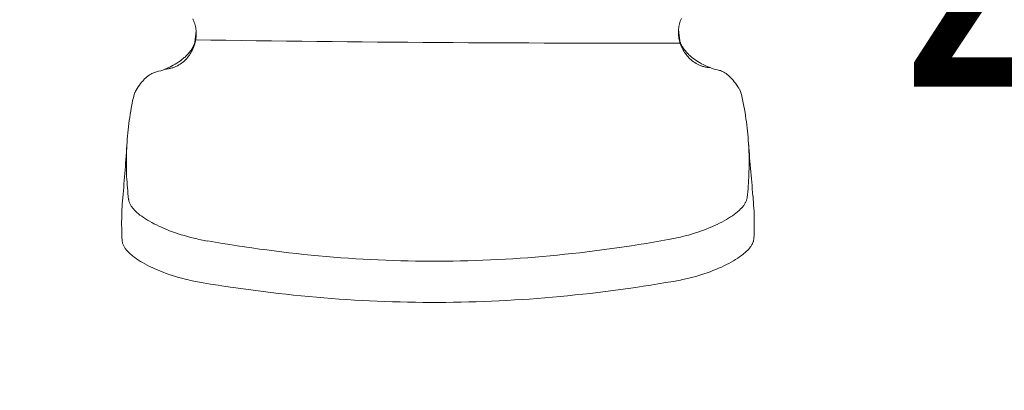
# Model space of a CAD drawing. Units: inches. Extents: x -466983 to 1020, y 324 to 318697.
# Tile 35 of 97: x 867.6 to 887.72, y 734.38 to 741.96. Entities that reach past the tile are written whole.
import ezdxf

# ---------------------------------------------------------------- set-up
doc = ezdxf.new("R2010")
doc.units = ezdxf.units.IN
doc.header["$MEASUREMENT"] = 0
for name, color, linetype, lineweight in [('A-ANNO-DIMS', 2, 'Continuous', 18), ('A-FLOR-PATT', 252, 'Continuous', 13), ('A-FURN', 8, 'Continuous', 18)]:
    doc.layers.add(name, color=color, linetype=linetype, lineweight=lineweight)
doc.styles.get("Standard").update_dxf_attribs({"font": 'arial.ttf'})
doc.dimstyles.get("Standard").update_dxf_attribs({"dimtxt": 6, "dimasz": 4, "dimexe": 3, "dimexo": 3, "dimgap": 0.09, "dimtad": 0, "dimtih": 1, "dimtoh": 1, "dimdec": 1, "dimzin": 0, "dimdsep": 46, "dimlunit": 3, "dimtxsty": 'Standard', "dimcen": 0.09, "dimadec": 0, "dimazin": 0, "dimtfac": 1, "dimtdec": 1, "dimtofl": 0, "dimtmove": 0, "dimatfit": 3, "dimfxl": 1, "dimtolj": 1, "dimtzin": 0, "dimarcsym": 0})

# ---------------------------------------------------------------- blocks, each defined once
blk = doc.blocks.new('Office Chairs')
at = {"ltscale": 60}
for p, q in [((3701, 927.5), (3701.6, 926.1)), ((3701.6, 926.1), (3702.2, 924.7)), ((3702.2, 924.7), (3702.7, 923.3)), ((3702.7, 923.3), (3703.2, 921.9)), ((4219.7, 923.5), (4219.4, 922.1)), ((4220.2, 924.9), (4219.7, 923.5)), ((4220.7, 926.3), (4220.2, 924.9)), ((4221.3, 927.7), (4220.7, 926.3)), ((3703.2, 921.9), (3703.6, 920.5)), ((3703.6, 920.5), (3703.9, 919.1)), ((3703.9, 919.1), (3704.2, 917.7)), ((3704.2, 917.7), (3704.4, 916.2)), ((3704.4, 916.2), (3704.6, 914.8)), ((3704.6, 914.8), (3704.7, 913.4)), ((3704.7, 913.8), (3704.7, 909.7)), ((3704.7, 913.4), (3704.7, 912)), ((4218.3, 914.9), (4218.2, 913.5)), ((4218.2, 913.5), (4218.2, 912.8)), ((4218.2, 912.8), (4218.2, 912.7)), ((4218.4, 916.4), (4218.3, 914.9)), ((4218.3, 915.2), (4218.3, 911.3)), ((4218.5, 917.8), (4218.4, 916.4)), ((4218.8, 919.2), (4218.5, 917.8)), ((4219, 920.7), (4218.8, 919.2)), ((4219.4, 922.1), (4219, 920.7)), ((3703, 901.2), (3703.2, 902.1)), ((3703.2, 902.1), (3703.2, 902.3)), ((3703.2, 902.3), (3703.2, 902.3)), ((3703.3, 900.6), (3703.6, 902.1)), ((3703.6, 902.1), (3704, 903.5)), ((3704, 903.5), (3704.2, 904.9)), ((3704.2, 904.9), (3704.4, 906.4)), ((3704.4, 906.4), (3704.6, 907.9)), ((3704.6, 907.9), (3704.7, 908.6)), ((3704.7, 912), (3704.8, 911.2)), ((3704.7, 909.7), (3704.7, 908.6)), ((4218.3, 911.3), (4218.3, 910.2)), ((4218.4, 909.4), (4218.3, 910.2)), ((4218.6, 908), (4218.4, 909.4)), ((4218.8, 906.5), (4218.6, 908)), ((4219.1, 905.1), (4218.8, 906.5)), ((4219.4, 903.6), (4219.1, 905.1)), ((4219.8, 902.2), (4219.4, 903.6)), ((4219.8, 903.7), (4219.8, 904)), ((4219.8, 904), (4219.8, 904)), ((4220, 902.8), (4219.8, 903.7)), ((4220.2, 900.8), (4219.8, 902.2)), ((4220.3, 901.9), (4220, 902.8)), ((4220.5, 901.4), (4220.3, 901.9)), ((3697.4, 891.4), (3696.7, 890.6)), ((3698.1, 892.3), (3697.4, 891.4)), ((3698.8, 893.2), (3698.1, 892.3)), ((3698.4, 890), (3699.2, 891.2)), ((3699.4, 894), (3698.8, 893.2)), ((3699.2, 891.2), (3699.9, 892.5)), ((3700, 895), (3699.4, 894)), ((3699.9, 892.5), (3700.6, 893.8)), ((3700.6, 895.9), (3700, 895)), ((3701.1, 896.8), (3700.6, 895.9)), ((3700.6, 893.8), (3701.2, 895.1)), ((3701.6, 897.8), (3701.1, 896.8)), ((3701.2, 895.1), (3701.8, 896.5)), ((3702.1, 898.8), (3701.6, 897.8)), ((3701.8, 896.5), (3702.3, 897.9)), ((3702.6, 899.8), (3702.1, 898.8)), ((3702.3, 897.9), (3702.8, 899.2)), ((3702.6, 899.8), (3702.7, 900.3)), ((3702.7, 900.3), (3703, 901.2)), ((3702.8, 899.2), (3703.3, 900.6)), ((4220.7, 899.4), (4220.2, 900.8)), ((4220.5, 901.4), (4220.9, 900.4)), ((4221.3, 898.1), (4220.7, 899.4)), ((4220.9, 900.4), (4221.4, 899.4)), ((4221.9, 896.7), (4221.3, 898.1)), ((4221.4, 899.4), (4221.9, 898.4)), ((4221.9, 898.4), (4222.5, 897.5)), ((4222.5, 895.4), (4221.9, 896.7)), ((4222.5, 897.5), (4223.1, 896.6)), ((4223.2, 894.1), (4222.5, 895.4)), ((4223.1, 896.6), (4223.7, 895.7)), ((4223.9, 892.8), (4223.2, 894.1)), ((4223.7, 895.7), (4224.3, 894.8)), ((4224.7, 891.6), (4223.9, 892.8)), ((4224.3, 894.8), (4225, 893.9)), ((4225.6, 890.4), (4224.7, 891.6)), ((4225, 893.9), (4225.7, 893.1)), ((4225.7, 893.1), (4226.4, 892.2)), ((4226.4, 892.2), (4227.1, 891.4)), ((4227.1, 891.4), (4227.9, 890.6)), ((3686.1, 881.4), (3684.2, 880.2)), ((3687.9, 882.6), (3686.1, 881.4)), ((3689.6, 883.9), (3687.9, 882.6)), ((3689, 880), (3690.3, 881)), ((3691.3, 885.3), (3689.6, 883.9)), ((3690.3, 881), (3691.5, 882)), ((3692.1, 886), (3691.3, 885.3)), ((3691.5, 882), (3692.6, 883)), ((3692.9, 886.7), (3692.1, 886)), ((3692.6, 883), (3693.7, 884.1)), ((3693.7, 887.5), (3692.9, 886.7)), ((3694.5, 888.2), (3693.7, 887.5)), ((3693.7, 884.1), (3694.8, 885.2)), ((3695.3, 889), (3694.5, 888.2)), ((3694.8, 885.2), (3695.8, 886.4)), ((3696, 889.8), (3695.3, 889)), ((3695.8, 886.4), (3696.7, 887.6)), ((3696.7, 890.6), (3696, 889.8)), ((3696.7, 887.6), (3697.6, 888.8)), ((3697.6, 888.8), (3698.4, 890)), ((4226.4, 889.2), (4225.6, 890.4)), ((4227.4, 888), (4226.4, 889.2)), ((4228.4, 886.9), (4227.4, 888)), ((4227.9, 890.6), (4228.6, 889.9)), ((4229.4, 885.7), (4228.4, 886.9)), ((4228.6, 889.9), (4229.4, 889.1)), ((4229.4, 889.1), (4230.2, 888.4)), ((4230.5, 884.7), (4229.4, 885.7)), ((4230.2, 888.4), (4231, 887.7)), ((4231.7, 883.6), (4230.5, 884.7)), ((4231, 887.7), (4231.8, 887)), ((4232.9, 882.6), (4231.7, 883.6)), ((4231.8, 887), (4233.5, 885.6)), ((4234.2, 881.7), (4232.9, 882.6)), ((4233.5, 885.6), (4235.3, 884.3)), ((4235.6, 880.7), (4234.2, 881.7)), ((4235.3, 884.3), (4237.1, 883)), ((4237, 879.9), (4235.6, 880.7)), ((4237.1, 883), (4238.9, 881.8)), ((4238.9, 881.8), (4240.8, 880.7)), ((4240.8, 880.7), (4242.7, 879.6)), ((3659.3, 870), (3660.3, 870.3)), ((3660.3, 870.3), (3661.4, 870.7)), ((3661.4, 870.7), (3662.5, 871)), ((3662.5, 871), (3662.5, 871)), ((3672.4, 874.1), (3671.4, 873.7)), ((3671.4, 873.7), (3672.4, 873.8)), ((3674.5, 875), (3672.4, 874.1)), ((3672.4, 873.8), (3673.3, 873.9)), ((3673.3, 873.9), (3674.3, 874)), ((3674.3, 874), (3675.3, 874.1)), ((3676.5, 875.9), (3674.5, 875)), ((3675.3, 874.1), (3676.2, 874.3)), ((3676.2, 874.3), (3677.2, 874.5)), ((3678.5, 876.9), (3676.5, 875.9)), ((3677.2, 874.5), (3678.1, 874.8)), ((3678.1, 874.8), (3679, 875)), ((3680.4, 877.9), (3678.5, 876.9)), ((3679, 875), (3679.9, 875.3)), ((3679.9, 875.3), (3680.7, 875.6)), ((3682.4, 879), (3680.4, 877.9)), ((3680.7, 875.6), (3681.6, 875.9)), ((3681.6, 875.9), (3682.4, 876.3)), ((3684.2, 880.2), (3682.4, 879)), ((3682.4, 876.3), (3683.2, 876.6)), ((3683.2, 876.6), (3684, 877)), ((3684, 877), (3684.7, 877.4)), ((3684.7, 877.4), (3686.2, 878.2)), ((3686.2, 878.2), (3687.6, 879.1)), ((3687.6, 879.1), (3689, 880)), ((4238.5, 879.1), (4237, 879.9)), ((4239.2, 878.7), (4238.5, 879.1)), ((4240, 878.3), (4239.2, 878.7)), ((4240.8, 878), (4240, 878.3)), ((4241.6, 877.6), (4240.8, 878)), ((4242.5, 877.3), (4241.6, 877.6)), ((4243.4, 877), (4242.5, 877.3)), ((4242.7, 879.6), (4244.7, 878.6)), ((4244.2, 876.7), (4243.4, 877)), ((4245.1, 876.5), (4244.2, 876.7)), ((4244.7, 878.6), (4246.7, 877.6)), ((4246.1, 876.3), (4245.1, 876.5)), ((4247, 876), (4246.1, 876.3)), ((4246.7, 877.6), (4248.7, 876.7)), ((4247.9, 875.9), (4247, 876)), ((4248.9, 875.7), (4247.9, 875.9)), ((4248.7, 876.7), (4250.8, 875.9)), ((4249.9, 875.6), (4248.9, 875.7)), ((4250.9, 875.5), (4249.9, 875.6)), ((4250.8, 875.9), (4251.8, 875.5)), ((4251.8, 875.5), (4250.9, 875.5)), ((4260.8, 872.8), (4260.8, 872.8)), ((4261.9, 872.5), (4260.8, 872.8)), ((4262.9, 872.2), (4261.9, 872.5)), ((4263.9, 871.8), (4262.9, 872.2)), ((4264.9, 871.4), (4263.9, 871.8)), ((4265.8, 870.9), (4264.9, 871.4)), ((4266.6, 870.5), (4265.8, 870.9)), ((4267.5, 870), (4266.6, 870.5)), ((3645.6, 858.5), (3646.9, 860.1)), ((3646.9, 860.1), (3647.8, 861.1)), ((3647.8, 861.1), (3648.8, 862.2)), ((3648.8, 862.2), (3649.8, 863.3)), ((3649.8, 863.3), (3651, 864.4)), ((3651, 864.4), (3652.2, 865.5)), ((3652.2, 865.5), (3652.9, 866.1)), ((3652.9, 866.1), (3653.5, 866.6)), ((3653.5, 866.6), (3654.3, 867.1)), ((3654.3, 867.1), (3655, 867.6)), ((3655, 867.6), (3655.8, 868.1)), ((3655.8, 868.1), (3656.6, 868.6)), ((3656.6, 868.6), (3657.5, 869.1)), ((3657.5, 869.1), (3658.4, 869.5)), ((3658.4, 869.5), (3659.3, 870)), ((4268.3, 869.5), (4267.5, 870)), ((4269, 869), (4268.3, 869.5)), ((4269.7, 868.5), (4269, 869)), ((4270.4, 867.9), (4269.7, 868.5)), ((4271.1, 867.4), (4270.4, 867.9)), ((4272.3, 866.3), (4271.1, 867.4)), ((4273.4, 865.2), (4272.3, 866.3)), ((4274.5, 864.1), (4273.4, 865.2)), ((4275.5, 863), (4274.5, 864.1)), ((4276.4, 862), (4275.5, 863)), ((4277.7, 860.4), (4276.4, 862)), ((4278.9, 858.9), (4277.7, 860.4)), ((3640.1, 850.2), (3640, 850.1)), ((3640.1, 850.2), (3640.8, 851.4)), ((3640.8, 851.4), (3641.9, 853.1)), ((3641.9, 853.1), (3643.1, 855)), ((3643.1, 855), (3644.5, 856.9)), ((3644.5, 856.9), (3645.6, 858.5)), ((4280.3, 856.9), (4278.9, 858.9)), ((4281.5, 855.1), (4280.3, 856.9)), ((4282.6, 853.4), (4281.5, 855.1)), ((4283.3, 852.2), (4282.6, 853.4)), ((4283.3, 852.2), (4283.3, 852)), ((3634.5, 825.7), (3635, 829)), ((3635, 829), (3635.6, 832.3)), ((4288.5, 831), (4287.9, 834.3)), ((4289.1, 827.7), (4288.5, 831)), ((3633, 815.8), (3633.5, 819.1)), ((3633.5, 819.1), (3634, 822.4)), ((3634, 822.4), (3634.5, 825.7)), ((4289.6, 824.3), (4289.1, 827.7)), ((4290.1, 821), (4289.6, 824.3)), ((4290.6, 817.7), (4290.1, 821)), ((4291, 814.4), (4290.6, 817.7)), ((3631.9, 805.9), (3632.3, 809.2)), ((3632.3, 809.2), (3632.6, 812.5)), ((3632.6, 812.5), (3633, 815.8)), ((4291.4, 811.1), (4291, 814.4)), ((4291.8, 807.8), (4291.4, 811.1)), ((4292.1, 804.5), (4291.8, 807.8)), ((3631.1, 796), (3631.3, 799.3)), ((3631.3, 799.3), (3631.6, 802.6)), ((3631.6, 802.6), (3631.9, 805.9)), ((4292.4, 801.2), (4292.1, 804.5)), ((4292.6, 797.9), (4292.4, 801.2)), ((4292.8, 794.9), (4292.6, 797.9)), ((3630.5, 783.9), (3630.6, 787)), ((3630.6, 787), (3630.8, 790)), ((3630.8, 790), (3630.9, 793)), ((3630.9, 793), (3631.1, 796)), ((4293, 791.9), (4292.8, 794.9)), ((4293.2, 788.9), (4293, 791.9)), ((4293.3, 785.8), (4293.2, 788.9)), ((3630.4, 780.9), (3630.5, 783.9)), ((3630.4, 777.9), (3630.4, 780.9)), ((3630.4, 774.8), (3630.4, 777.9)), ((4293.4, 782.8), (4293.3, 785.8)), ((4293.5, 779.8), (4293.4, 782.8)), ((4293.5, 776.8), (4293.5, 779.8)), ((4293.5, 773.7), (4293.5, 776.8)), ((3630.4, 771.8), (3630.4, 774.8)), ((3630.4, 768.8), (3630.4, 771.8)), ((3630.5, 765.7), (3630.4, 768.8)), ((3630.6, 762.7), (3630.5, 765.7)), ((4293.3, 764.6), (4293.4, 767.7)), ((4293.4, 767.7), (4293.5, 770.7)), ((4293.5, 770.7), (4293.5, 773.7)), ((3630.7, 759.6), (3630.6, 762.7)), ((3630.9, 756.6), (3630.7, 759.6)), ((3631.1, 753.5), (3630.9, 756.6)), ((4292.7, 752.5), (4292.9, 755.5)), ((4292.9, 755.5), (4293.1, 758.6)), ((4293.1, 758.6), (4293.2, 761.6)), ((4293.2, 761.6), (4293.3, 764.6)), ((3631.3, 750.5), (3631.1, 753.5)), ((3631.5, 747.4), (3631.3, 750.5)), ((3631.8, 744.4), (3631.5, 747.4)), ((3632.1, 741.3), (3631.8, 744.4)), ((4292, 743.3), (4292.3, 746.3)), ((4292.3, 746.3), (4292.5, 749.4)), ((4292.5, 749.4), (4292.7, 752.5)), ((3626.3, 733.6), (3626.5, 736.8)), ((3632.4, 738.2), (3632.1, 741.3)), ((3632.8, 735.1), (3632.4, 738.2)), ((3632.8, 735.1), (3632.9, 734.5)), ((3632.9, 734.5), (3633, 733.9)), ((3633, 733.9), (3633.1, 733.2)), ((4290.6, 734), (4290.3, 733.3)), ((4290.8, 734.6), (4290.6, 734)), ((4291, 735.2), (4290.8, 734.6)), ((4291.2, 735.9), (4291, 735.2)), ((4291.3, 736.5), (4291.2, 735.9)), ((4291.4, 737.1), (4291.3, 736.5)), ((4291.4, 737.1), (4291.7, 740.2)), ((4291.7, 740.2), (4292, 743.3)), ((4297.9, 735.5), (4297.6, 738.7)), ((4298.1, 732.3), (4297.9, 735.5)), ((3625.5, 720.8), (3625.7, 724)), ((3625.7, 724), (3625.8, 727.2)), ((3625.8, 727.2), (3626, 730.4)), ((3626, 730.4), (3626.3, 733.6)), ((3633.1, 733.2), (3633.3, 732.6)), ((3633.3, 732.6), (3633.6, 732)), ((3633.6, 732), (3633.8, 731.3)), ((3633.8, 731.3), (3634.1, 730.7)), ((3634.1, 730.7), (3634.4, 730)), ((3634.4, 730), (3634.8, 729.3)), ((3634.8, 729.3), (3635.2, 728.7)), ((3635.2, 728.7), (3635.6, 728)), ((3635.6, 728), (3636.1, 727.3)), ((3636.1, 727.3), (3636.5, 726.7)), ((3636.5, 726.7), (3637.1, 726)), ((3637.1, 726), (3637.6, 725.3)), ((3637.6, 725.3), (3638.2, 724.7)), ((3638.2, 724.7), (3638.8, 724)), ((3638.8, 724), (3639.5, 723.3)), ((4283.4, 723.9), (4282.7, 723.2)), ((4284.1, 724.6), (4283.4, 723.9)), ((4284.8, 725.3), (4284.1, 724.6)), ((4285.4, 725.9), (4284.8, 725.3)), ((4286, 726.6), (4285.4, 725.9)), ((4286.6, 727.3), (4286, 726.6)), ((4287.1, 728), (4286.6, 727.3)), ((4287.7, 728.7), (4287.1, 728)), ((4288.1, 729.3), (4287.7, 728.7)), ((4288.6, 730), (4288.1, 729.3)), ((4289, 730.7), (4288.6, 730)), ((4289.4, 731.3), (4289, 730.7)), ((4289.7, 732), (4289.4, 731.3)), ((4290.1, 732.7), (4289.7, 732)), ((4290.3, 733.3), (4290.1, 732.7)), ((4298.3, 729.1), (4298.1, 732.3)), ((4298.5, 725.9), (4298.3, 729.1)), ((4298.7, 722.7), (4298.5, 725.9)), ((3625.3, 711.1), (3625.4, 714.3)), ((3625.4, 717.5), (3625.5, 720.8)), ((3625.4, 714.3), (3625.4, 717.5)), ((3639.5, 723.3), (3640.1, 722.6)), ((3640.1, 722.6), (3640.8, 721.9)), ((3640.8, 721.9), (3641.6, 721.3)), ((3641.6, 721.3), (3643.2, 719.9)), ((3643.2, 719.9), (3644.8, 718.5)), ((3644.8, 718.5), (3646.7, 717.2)), ((3646.7, 717.2), (3648.6, 715.8)), ((3648.6, 715.8), (3650.6, 714.5)), ((3650.6, 714.5), (3652.8, 713.1)), ((3652.8, 713.1), (3655, 711.8)), ((4269.3, 713.7), (4266.9, 712.3)), ((4271.5, 715), (4269.3, 713.7)), ((4273.7, 716.4), (4271.5, 715)), ((4275.7, 717.7), (4273.7, 716.4)), ((4277.6, 719.1), (4275.7, 717.7)), ((4279.4, 720.5), (4277.6, 719.1)), ((4281.1, 721.8), (4279.4, 720.5)), ((4282.7, 723.2), (4281.1, 721.8)), ((4298.8, 719.5), (4298.7, 722.7)), ((4298.9, 716.3), (4298.8, 719.5)), ((4298.9, 713.1), (4298.9, 716.3)), ((4299, 709.8), (4298.9, 713.1)), ((3625.3, 707.9), (3625.3, 711.1)), ((3625.4, 704.6), (3625.3, 707.9)), ((3625.4, 701.4), (3625.4, 704.6)), ((3655, 711.8), (3657.4, 710.5)), ((3657.4, 710.5), (3659.8, 709.2)), ((3659.8, 709.2), (3662.4, 707.9)), ((3662.4, 707.9), (3665, 706.6)), ((3665, 706.6), (3667.7, 705.4)), ((3667.7, 705.4), (3670.6, 704.2)), ((3670.6, 704.2), (3673.5, 703)), ((3673.5, 703), (3676.4, 701.8)), ((4244.9, 702.4), (4241.8, 701.3)), ((4247.9, 703.6), (4244.9, 702.4)), ((4250.9, 704.7), (4247.9, 703.6)), ((4253.8, 705.9), (4250.9, 704.7)), ((4256.6, 707.2), (4253.8, 705.9)), ((4259.3, 708.4), (4256.6, 707.2)), ((4261.9, 709.7), (4259.3, 708.4)), ((4264.5, 711), (4261.9, 709.7)), ((4266.9, 712.3), (4264.5, 711)), ((4298.8, 700.2), (4298.9, 703.4)), ((4298.9, 703.4), (4299, 706.6)), ((4299, 706.6), (4299, 709.8)), ((3625.5, 698.1), (3625.4, 701.4)), ((3625.7, 694.9), (3625.5, 698.1)), ((3625.8, 691.6), (3625.7, 694.9)), ((3676.4, 701.8), (3679.5, 700.7)), ((3679.5, 700.7), (3682.6, 699.6)), ((3682.6, 699.6), (3685.7, 698.6)), ((3685.7, 698.6), (3688.9, 697.5)), ((3688.9, 697.5), (3692.2, 696.6)), ((3692.2, 696.6), (3695.5, 695.6)), ((3695.5, 695.6), (3698.9, 694.7)), ((3698.9, 694.7), (3702.3, 693.9)), ((4199.6, 691), (4207.4, 692.3)), ((4225.5, 696.3), (4222.1, 695.5)), ((4228.9, 697.2), (4225.5, 696.3)), ((4232.2, 698.2), (4228.9, 697.2)), ((4235.4, 699.2), (4232.2, 698.2)), ((4238.7, 700.2), (4235.4, 699.2)), ((4241.8, 701.3), (4238.7, 700.2)), ((4298.3, 691.7), (4298.4, 692.4)), ((4298.4, 692.4), (4298.5, 693)), ((4298.5, 693), (4298.6, 693.7)), ((4298.6, 693.7), (4298.7, 696.9)), ((4298.7, 696.9), (4298.8, 700.2)), ((3625.9, 691), (3625.8, 691.6)), ((3626, 690.4), (3625.9, 691)), ((3626.1, 689.7), (3626, 690.4)), ((3626.2, 689), (3626.1, 689.7)), ((3626.4, 688.4), (3626.2, 689)), ((3626.7, 687.7), (3626.4, 688.4)), ((3626.9, 687.1), (3626.7, 687.7)), ((3627.2, 686.4), (3626.9, 687.1)), ((3627.6, 685.7), (3627.2, 686.4)), ((3627.9, 685), (3627.6, 685.7)), ((3628.3, 684.4), (3627.9, 685)), ((3628.8, 683.7), (3628.3, 684.4)), ((3629.2, 683), (3628.8, 683.7)), ((3629.7, 682.3), (3629.2, 683)), ((3630.3, 681.6), (3629.7, 682.3)), ((3630.8, 680.9), (3630.3, 681.6)), ((3724.8, 689.5), (3717, 690.9)), ((3732.7, 688.2), (3724.8, 689.5)), ((3740.5, 687), (3732.7, 688.2)), ((3748.4, 685.7), (3740.5, 687)), ((3756.2, 684.6), (3748.4, 685.7)), ((3764.1, 683.4), (3756.2, 684.6)), ((3772, 682.3), (3764.1, 683.4)), ((3779.8, 681.3), (3772, 682.3)), ((4136.8, 681.3), (4144.7, 682.4)), ((4144.7, 682.4), (4152.5, 683.5)), ((4152.5, 683.5), (4160.4, 684.6)), ((4160.4, 684.6), (4168.3, 685.8)), ((4168.3, 685.8), (4176.1, 687)), ((4176.1, 687), (4184, 688.3)), ((4184, 688.3), (4191.8, 689.6)), ((4191.8, 689.6), (4199.6, 691)), ((4291.7, 680.9), (4292.4, 681.6)), ((4292.4, 681.6), (4293, 682.3)), ((4293, 682.3), (4293.6, 682.9)), ((4293.6, 682.9), (4294.2, 683.6)), ((4294.2, 683.6), (4294.7, 684.3)), ((4294.7, 684.3), (4295.2, 685)), ((4295.2, 685), (4295.7, 685.7)), ((4295.7, 685.7), (4296.1, 686.4)), ((4296.1, 686.4), (4296.5, 687.1)), ((4296.5, 687.1), (4296.9, 687.7)), ((4296.9, 687.7), (4297.2, 688.4)), ((4297.2, 688.4), (4297.5, 689.1)), ((4297.5, 689.1), (4297.8, 689.8)), ((4297.8, 689.8), (4298, 690.4)), ((4298, 690.4), (4298.2, 691.1)), ((4298.2, 691.1), (4298.3, 691.7)), ((3631.4, 680.2), (3630.8, 680.9)), ((3632.1, 679.5), (3631.4, 680.2)), ((3632.7, 678.9), (3632.1, 679.5)), ((3633.4, 678.2), (3632.7, 678.9)), ((3634.2, 677.5), (3633.4, 678.2)), ((3634.9, 676.8), (3634.2, 677.5)), ((3635.7, 676.1), (3634.9, 676.8)), ((3636.6, 675.4), (3635.7, 676.1)), ((3637.4, 674.7), (3636.6, 675.4)), ((3639.3, 673.3), (3637.4, 674.7)), ((3641.2, 671.9), (3639.3, 673.3)), ((3643.2, 670.5), (3641.2, 671.9)), ((3787.7, 680.3), (3779.8, 681.3)), ((3795.6, 679.3), (3787.7, 680.3)), ((3803.5, 678.4), (3795.6, 679.3)), ((3811.4, 677.5), (3803.5, 678.4)), ((3819.3, 676.6), (3811.4, 677.5)), ((3827.2, 675.8), (3819.3, 676.6)), ((3835.1, 675.1), (3827.2, 675.8)), ((3843.1, 674.4), (3835.1, 675.1)), ((3851, 673.7), (3843.1, 674.4)), ((3858.9, 673.1), (3851, 673.7)), ((3866.9, 672.5), (3858.9, 673.1)), ((3874.8, 672), (3866.9, 672.5)), ((3882.7, 671.5), (3874.8, 672)), ((3890.7, 671.1), (3882.7, 671.5)), ((3898.6, 670.7), (3890.7, 671.1)), ((4018, 670.7), (4025.9, 671.1)), ((4025.9, 671.1), (4033.9, 671.5)), ((4033.9, 671.5), (4041.8, 672)), ((4041.8, 672), (4049.7, 672.5)), ((4049.7, 672.5), (4057.7, 673.1)), ((4057.7, 673.1), (4065.6, 673.7)), ((4065.6, 673.7), (4073.5, 674.4)), ((4073.5, 674.4), (4081.5, 675.1)), ((4081.5, 675.1), (4089.4, 675.9)), ((4089.4, 675.9), (4097.3, 676.7)), ((4097.3, 676.7), (4105.2, 677.5)), ((4105.2, 677.5), (4113.1, 678.4)), ((4113.1, 678.4), (4121, 679.3)), ((4121, 679.3), (4128.9, 680.3)), ((4128.9, 680.3), (4136.8, 681.3)), ((4276.9, 669.7), (4279.1, 671.1)), ((4279.1, 671.1), (4281.3, 672.5)), ((4281.3, 672.5), (4283.3, 673.9)), ((4283.3, 673.9), (4285.3, 675.3)), ((4285.3, 675.3), (4287.1, 676.7)), ((4287.1, 676.7), (4287.9, 677.4)), ((4287.9, 677.4), (4288.8, 678.1)), ((4288.8, 678.1), (4289.6, 678.8)), ((4289.6, 678.8), (4290.3, 679.5)), ((4290.3, 679.5), (4291, 680.2)), ((4291, 680.2), (4291.7, 680.9)), ((3645.4, 669.1), (3643.2, 670.5)), ((3647.7, 667.8), (3645.4, 669.1)), ((3650.1, 666.4), (3647.7, 667.8)), ((3652.6, 665.1), (3650.1, 666.4)), ((3655.2, 663.8), (3652.6, 665.1)), ((3657.9, 662.5), (3655.2, 663.8)), ((3660.7, 661.2), (3657.9, 662.5)), ((3663.6, 660), (3660.7, 661.2)), ((3906.6, 670.4), (3898.6, 670.7)), ((3914.5, 670.1), (3906.6, 670.4)), ((3922.5, 669.9), (3914.5, 670.1)), ((3930.5, 669.7), (3922.5, 669.9)), ((3938.4, 669.5), (3930.5, 669.7)), ((3946.4, 669.4), (3938.4, 669.5)), ((3954.3, 669.4), (3946.4, 669.4)), ((3962.3, 669.4), (3954.3, 669.4)), ((3962.3, 669.4), (3970.2, 669.4)), ((3970.2, 669.4), (3978.2, 669.5)), ((3978.2, 669.5), (3986.2, 669.7)), ((3986.2, 669.7), (3994.1, 669.9)), ((3994.1, 669.9), (4002.1, 670.1)), ((4002.1, 670.1), (4010, 670.4)), ((4010, 670.4), (4018, 670.7)), ((4255, 659.3), (4258.1, 660.5)), ((4258.1, 660.5), (4261, 661.8)), ((4261, 661.8), (4263.9, 663)), ((4263.9, 663), (4266.7, 664.3)), ((4266.7, 664.3), (4269.4, 665.7)), ((4269.4, 665.7), (4272, 667)), ((4272, 667), (4274.5, 668.3)), ((4274.5, 668.3), (4276.9, 669.7)), ((3666.6, 658.7), (3663.6, 660)), ((3669.6, 657.6), (3666.6, 658.7)), ((3672.8, 656.4), (3669.6, 657.6)), ((3676, 655.3), (3672.8, 656.4)), ((3679.2, 654.2), (3676, 655.3)), ((3682.6, 653.1), (3679.2, 654.2)), ((3686, 652.1), (3682.6, 653.1)), ((3689.4, 651.2), (3686, 652.1)), ((3692.9, 650.3), (3689.4, 651.2)), ((3696.5, 649.4), (3692.9, 650.3)), ((4228.2, 651), (4231.7, 651.9)), ((4231.7, 651.9), (4235.2, 652.8)), ((4235.2, 652.8), (4238.7, 653.8)), ((4238.7, 653.8), (4242.1, 654.8)), ((4242.1, 654.8), (4245.4, 655.9)), ((4245.4, 655.9), (4248.7, 657)), ((4248.7, 657), (4251.9, 658.2)), ((4251.9, 658.2), (4255, 659.3)), ((3720, 645), (3712, 646.3)), ((3728, 643.7), (3720, 645)), ((3736, 642.5), (3728, 643.7)), ((3744, 641.3), (3736, 642.5)), ((3752.1, 640.2), (3744, 641.3)), ((3760.1, 639.1), (3752.1, 640.2)), ((4156.6, 639.2), (4164.6, 640.3)), ((4164.6, 640.3), (4172.7, 641.5)), ((4172.7, 641.5), (4180.7, 642.7)), ((4180.7, 642.7), (4188.7, 643.9)), ((4188.7, 643.9), (4196.7, 645.2)), ((4196.7, 645.2), (4204.7, 646.5)), ((4204.7, 646.5), (4212.7, 647.8)), ((3768.1, 638), (3760.1, 639.1)), ((3776.2, 637), (3768.1, 638)), ((3784.2, 636), (3776.2, 637)), ((3792.3, 635.1), (3784.2, 636)), ((3800.4, 634.2), (3792.3, 635.1)), ((3808.4, 633.3), (3800.4, 634.2)), ((3816.5, 632.5), (3808.4, 633.3)), ((3824.6, 631.7), (3816.5, 632.5)), ((3832.7, 631), (3824.6, 631.7)), ((3840.8, 630.3), (3832.7, 631)), ((3848.9, 629.7), (3840.8, 630.3)), ((3857, 629.1), (3848.9, 629.7)), ((3865.1, 628.5), (3857, 629.1)), ((4051.7, 628.6), (4059.8, 629.1)), ((4059.8, 629.1), (4067.8, 629.7)), ((4067.8, 629.7), (4075.9, 630.4)), ((4075.9, 630.4), (4084, 631.1)), ((4084, 631.1), (4092.1, 631.8)), ((4092.1, 631.8), (4100.2, 632.6)), ((4100.2, 632.6), (4108.3, 633.4)), ((4108.3, 633.4), (4116.3, 634.2)), ((4116.3, 634.2), (4124.4, 635.1)), ((4124.4, 635.1), (4132.5, 636.1)), ((4132.5, 636.1), (4140.5, 637.1)), ((4140.5, 637.1), (4148.6, 638.1)), ((4148.6, 638.1), (4156.6, 639.2)), ((3873.2, 628), (3865.1, 628.5)), ((3881.3, 627.6), (3873.2, 628)), ((3889.4, 627.2), (3881.3, 627.6)), ((3897.5, 626.8), (3889.4, 627.2)), ((3905.6, 626.5), (3897.5, 626.8)), ((3913.7, 626.2), (3905.6, 626.5)), ((3921.8, 626), (3913.7, 626.2)), ((3929.9, 625.8), (3921.8, 626)), ((3938.1, 625.6), (3929.9, 625.8)), ((3946.2, 625.5), (3938.1, 625.6)), ((3954.3, 625.5), (3946.2, 625.5)), ((3962.4, 625.5), (3954.3, 625.5)), ((3962.4, 625.5), (3970.5, 625.5)), ((3970.5, 625.5), (3978.7, 625.6)), ((3978.7, 625.6), (3986.8, 625.8)), ((3986.8, 625.8), (3994.9, 626)), ((3994.9, 626), (4003, 626.2)), ((4003, 626.2), (4011.1, 626.5)), ((4011.1, 626.5), (4019.2, 626.8)), ((4019.2, 626.8), (4027.3, 627.2)), ((4027.3, 627.2), (4035.4, 627.6)), ((4035.4, 627.6), (4043.6, 628.1)), ((4043.6, 628.1), (4051.7, 628.6))]:
    blk.add_line(p, q, dxfattribs=at)
for centre, radius, start, end in [((3549.7, 925.9), 155.4, 351.2767, 355.7808), ((4256.2, 913), 38, 180.4457, 184.3253), ((4373.2, 928.4), 155.3, 184.596, 189.0363), ((3677.2, 910.5), 27.5, 337.0771, 356.0895), ((3666.8, 911.2), 38, 356.0263, 0.0045), ((4245.8, 912.2), 27.5, 184.2618, 203.2092), ((3645.4, 942.2), 73.3, 283.461, 290.752), ((4277.4, 944.1), 73.3, 249.5975, 256.8877), ((3663.3, 837.2), 26.5, 151.1039, 153.8842), ((4260.2, 839), 26.6, 26.4885, 29.266), ((4251.9, 837.3), 34.8, 19.2532, 23.0465), ((3925.9, 779.5), 295, 166.8237, 169.6939), ((3671.5, 835.5), 34.7, 157.3274, 161.1267), ((3997.9, 779.5), 295.1, 10.6893, 13.5585), ((7201.2, 1011.1), 2916.4, 184.1922, 185.3594), ((721.2, 991.2), 2916.5, 354.9968, 356.1633), ((3756.5, 919.3), 231.9, 256.4666, 260.1773), ((4166.5, 920.5), 231.8, 280.1709, 283.8822), ((4173.4, 877.4), 232.9, 279.7144, 283.5949), ((3749.9, 876.1), 232.9, 256.7538, 260.6338)]:
    blk.add_arc(centre, radius, start, end, dxfattribs=at)
blk.add_arc((4146.2, 29055.7), 28154.2, 269.10045, 270.15098)
blk = doc.blocks.new('Office Desk With Chairs')
at = {"xscale": 0.0191941550942558, "yscale": 0.0191941550942558, "zscale": 0.0191941550942558}
blk.add_blockref('Office Chairs', (2012.509, 1014.21), dxfattribs=at)
blk = doc.blocks.new('*D91')
at = {"layer": 'A-ANNO-DIMS', "color": 0, "lineweight": -2, "transparency": 16777216}
for p, q in [((938.253, 802.547), (920.07, 802.547)), ((923.07, 798.547), (923.07, 745.132)), ((923.07, 685.328), (923.07, 738.743)), ((938.253, 681.328), (920.07, 681.328))]:
    blk.add_line(p, q, dxfattribs=at)
at = {"layer": 'A-ANNO-DIMS', "color": 0, "transparency": 16777216}
for points in [[(922.404, 798.547), (923.737, 798.547), (923.07, 802.547)], [(922.404, 685.328), (923.737, 685.328), (923.07, 681.328)]]:
    blk.add_solid(points, dxfattribs=at)
at = {"layer": 'Defpoints', "color": 0, "transparency": 16777216}
for p in [(941.253, 802.547), (923.07, 681.328), (941.253, 681.328)]:
    blk.add_point(p, dxfattribs=at)
at = {"layer": 'A-ANNO-DIMS', "color": 0, "transparency": 16777216, "insert": (923.07, 741.937), "char_height": 6, "attachment_point": 5}
blk.add_mtext('\\A1;4-SEATER SOFA 121', dxfattribs=at)

msp = doc.modelspace()

# ---------------------------------------------------------------- hatches: boundary and pattern name
at = {"layer": 'A-FLOR-PATT', "transparency": 33554572}
h = msp.add_hatch(dxfattribs=at)
h.set_pattern_fill('ANSI37', color=256, scale=30)
h.set_pattern_definition([(45, (-1212.4137, -290.035), (-2.6516504, 2.6516504), []), (135, (-1212.4137, -290.035), (-2.6516504, -2.6516504), [])])
h.paths.add_polyline_path([(901.806, 1075.938), (900.614, 1075.938), (900.614, 1065.386), (899.391, 1065.386), (898.091, 1065.386), (892.836, 1058.71, -0.258377), (892.188, 1058.351), (879.985, 1058.351, -0.20177), (879.438, 1058.581), (874.081, 1065.386), (872.781, 1065.386), (871.558, 1065.386), (871.558, 1075.938), (813.806, 1075.938), (813.806, 1044.792), (832.395, 1044.792, -0.394795), (848.66, 1028.536), (848.66, 1009.938), (901.806, 1009.938), (901.806, 1015.938), (901.306, 1015.938), (871.306, 1015.938), (871.306, 1017.25), (871.334, 1017.25, -0.401453), (901.306, 1045.938), (901.806, 1045.938)])
edge = h.paths.add_edge_path(flags=16)
edge.add_line((847.773, 1068.949), (847.773, 1073.709))
edge.add_arc((849.227, 1073.709), 1.454, 90, 180, ccw=False)
edge.add_line((849.227, 1075.163), (864.492, 1075.163))
edge.add_arc((864.492, 1073.709), 1.454, 0, 90, ccw=False)
edge.add_line((865.946, 1073.709), (865.946, 1069.004))
edge.add_arc((832.645, 1068.976), 33.301, -20.6123, 0.0472, ccw=False)
edge.add_ellipse((856.859, 1058.48), major_axis=(0, 10.213), ratio=0.685919, start_angle=100.0088, end_angle=259.9912, ccw=False)
edge.add_arc((881.074, 1068.976), 33.301, 180.0472, 200.6123, ccw=False)
h.paths.add_polyline_path([(853.146, 1066.482), (853.146, 1066.453), (853.146, 1066.453, 0.433107), (852.917, 1066.685), (852.917, 1066.453), (853.146, 1066.453), (853.146, 1066.482), (853.088, 1066.612, 0.697939), (852.7, 1066.453), (852.7, 1066.453), (852.7, 1066.482), (852.917, 1067.001), (852.917, 1066.685, -0.396254)], flags=0)
h.paths.add_polyline_path([(861.019, 1066.482), (861.019, 1066.453), (861.019, 1066.453, 0.416404), (860.802, 1066.685), (860.802, 1066.453), (861.019, 1066.453), (861.019, 1066.482), (860.967, 1066.605, 0.713344), (860.573, 1066.453), (860.573, 1066.453), (860.573, 1066.482), (860.802, 1067.001), (860.802, 1066.685, -0.379973)], flags=0)
edge = h.paths.add_edge_path(flags=0)
edge.add_spline(control_points=[(861.13, 1065.785), (861.466, 1065.248), (861.613, 1065.016), (861.983, 1064.374), (862.192, 1063.944), (862.561, 1063.039), (862.721, 1062.563), (862.987, 1061.578), (863.092, 1061.069), (863.245, 1060.031), (863.293, 1059.503), (863.329, 1058.441), (863.318, 1057.908), (863.237, 1056.852), (863.166, 1056.329), (862.97, 1055.308), (862.843, 1054.81), (862.537, 1053.852), (862.357, 1053.393), (861.951, 1052.525), (861.725, 1052.117), (861.233, 1051.362), (860.967, 1051.016), (860.405, 1050.395), (860.108, 1050.12), (859.494, 1049.646), (859.176, 1049.448), (858.528, 1049.13), (858.197, 1049.011), (857.531, 1048.852), (857.196, 1048.812), (856.525, 1048.812), (856.189, 1048.852), (855.524, 1049.01), (855.193, 1049.129), (854.545, 1049.447), (854.227, 1049.645), (853.612, 1050.118), (853.316, 1050.393), (852.753, 1051.014), (852.487, 1051.36), (851.995, 1052.114), (851.769, 1052.523), (851.363, 1053.39), (851.183, 1053.85), (850.877, 1054.807), (850.75, 1055.305), (850.553, 1056.326), (850.483, 1056.849), (850.401, 1057.905), (850.39, 1058.438), (850.426, 1059.5), (850.473, 1060.028), (850.626, 1061.066), (850.732, 1061.575), (850.997, 1062.561), (851.157, 1063.036), (851.525, 1063.942), (851.734, 1064.371), (852.106, 1065.016), (852.254, 1065.25), (852.608, 1065.733)], knot_values=[3.915332, 3.915332, 3.915332, 3.915332, 4.013468, 4.013468, 4.175532, 4.175532, 4.337596, 4.337596, 4.49966, 4.49966, 4.661724, 4.661724, 4.823788, 4.823788, 4.985852, 4.985852, 5.147916, 5.147916, 5.30998, 5.30998, 5.472044, 5.472044, 5.634109, 5.634109, 5.796173, 5.796173, 5.958237, 5.958237, 6.120301, 6.120301, 6.282365, 6.282365, 6.444429, 6.444429, 6.606493, 6.606493, 6.768557, 6.768557, 6.930621, 6.930621, 7.092685, 7.092685, 7.254749, 7.254749, 7.416813, 7.416813, 7.578878, 7.578878, 7.740942, 7.740942, 7.903006, 7.903006, 8.06507, 8.06507, 8.227134, 8.227134, 8.389198, 8.389198, 8.551262, 8.551262, 8.65037, 8.65037, 8.65037, 8.65037], degree=3, periodic=0)
edge.add_line((852.642, 1065.785), (861.13, 1065.785))
edge = h.paths.add_edge_path(flags=0)
edge.add_ellipse((856.85, 1057.743), major_axis=(0, 7.792), ratio=0.687861, start_angle=0, end_angle=360)
h.paths.add_polyline_path([(848.863, 1069.389), (848.863, 1073.96, -0.414214), (849.954, 1075.051), (863.765, 1075.051, -0.414214), (864.856, 1073.96), (864.856, 1069.389, -0.388936), (864.524, 1069.027, -0.043561), (849.195, 1069.027, -0.388936)], flags=0)
h.paths.add_polyline_path([(853.101, 1068.112, -1), (852.677, 1068.112, -1)], flags=0)
edge = h.paths.add_edge_path(flags=0)
edge.add_ellipse((856.859, 1057.338), major_axis=(0, 2.207), ratio=0.657164, start_angle=0, end_angle=360)
h.paths.add_polyline_path([(861.041, 1068.112, -1), (860.618, 1068.112, -1)], flags=0)
edge = h.paths.add_edge_path()
edge.add_line((573.954, 1057.341), (573.954, 1075.938))
edge.add_line((573.954, 1075.938), (558.731, 1075.938))
edge.add_line((558.731, 1075.938), (558.731, 1065.386))
edge.add_line((558.731, 1065.386), (557.507, 1065.386))
edge.add_line((557.507, 1065.386), (556.207, 1065.386))
edge.add_line((556.207, 1065.386), (550.952, 1058.71))
edge.add_arc((550.304, 1059.116), 0.765, 270, 327.9483, ccw=False)
edge.add_line((550.304, 1058.351), (538.101, 1058.351))
edge.add_arc((538.101, 1059.116), 0.765, 224.3704, 270, ccw=False)
edge.add_line((537.555, 1058.581), (532.198, 1065.386))
edge.add_line((532.198, 1065.386), (530.898, 1065.386))
edge.add_line((530.898, 1065.386), (529.674, 1065.386))
edge.add_line((529.674, 1065.386), (529.674, 1075.938))
edge.add_line((529.674, 1075.938), (520.806, 1075.938))
edge.add_line((520.806, 1075.938), (520.806, 1045.938))
edge.add_line((520.806, 1045.938), (521.306, 1045.938))
edge.add_arc((521.306, 1015.938), 30, 2.5075, 90, ccw=False)
edge.add_line((551.277, 1017.25), (551.306, 1017.25))
edge.add_line((551.306, 1017.25), (551.306, 1015.938))
edge.add_line((551.306, 1015.938), (520.806, 1015.938))
edge.add_line((520.806, 1015.938), (520.806, 1009.938))
edge.add_line((520.806, 1009.938), (559.191, 1010.402))
edge.add_arc((559.191, 1011.856), 1.454, 180, 270, ccw=False)
edge.add_line((557.737, 1011.856), (557.737, 1016.561))
edge.add_arc((591.039, 1016.589), 33.301, 159.3877, 180.0472, ccw=False)
edge.add_ellipse((566.824, 1027.085), major_axis=(0, 10.213), ratio=0.685919, start_angle=280.0088, end_angle=439.9912, ccw=False)
edge.add_arc((542.609, 1016.589), 33.301, 0.0472, 20.6123, ccw=False)
edge.add_line((575.91, 1016.616), (575.91, 1011.856))
edge.add_arc((574.456, 1011.856), 1.454, -90, 0, ccw=False)
edge.add_line((574.456, 1010.402), (608.806, 1009.938))
edge.add_line((608.806, 1009.938), (608.806, 1041.086))
edge.add_line((608.806, 1041.086), (590.218, 1041.086))
edge.add_arc((590.775, 1057.907), 16.831, 181.9277, 268.1032, ccw=False)
edge = h.paths.add_edge_path()
edge.add_ellipse((494.244, 583.62), major_axis=(0, 10.213), ratio=0.685919, start_angle=280.0088, end_angle=439.9912, ccw=False)
edge.add_arc((470.03, 573.124), 33.301, 0.0472, 20.6123, ccw=False)
edge.add_line((503.331, 573.152), (503.331, 568.392))
edge.add_arc((501.877, 568.392), 1.454, -90, 0, ccw=False)
edge.add_line((501.877, 566.938), (539.806, 566.938))
edge.add_line((539.806, 566.938), (539.806, 572.938))
edge.add_line((539.806, 572.938), (539.306, 572.938))
edge.add_line((539.306, 572.938), (509.306, 572.938))
edge.add_line((509.306, 572.938), (509.306, 574.25))
edge.add_line((509.306, 574.25), (509.334, 574.25))
edge.add_arc((539.306, 572.938), 30, 90, 177.4925, ccw=False)
edge.add_line((539.306, 602.938), (539.806, 602.938))
edge.add_line((539.806, 602.938), (539.806, 626.938))
edge.add_line((539.806, 626.938), (531.772, 626.938))
edge.add_line((531.772, 626.938), (531.772, 616.386))
edge.add_line((531.772, 616.386), (530.548, 616.386))
edge.add_line((530.548, 616.386), (529.249, 616.386))
edge.add_line((529.249, 616.386), (523.711, 609.351))
edge.add_line((523.711, 609.351), (510.777, 609.351))
edge.add_line((510.777, 609.351), (505.239, 616.386))
edge.add_line((505.239, 616.386), (503.939, 616.386))
edge.add_line((503.939, 616.386), (502.715, 616.386))
edge.add_line((502.715, 616.386), (502.715, 626.938))
edge.add_line((502.715, 626.938), (481.698, 626.938))
edge.add_line((481.698, 626.938), (481.698, 610.995))
edge.add_arc((467.27, 611.473), 14.436, 271.9277, 358.1032, ccw=False)
edge.add_line((467.756, 597.045), (451.806, 597.045))
edge.add_line((451.806, 597.045), (451.806, 584.404))
edge.add_line((451.806, 584.404), (451.806, 566.938))
edge.add_line((451.806, 566.938), (486.612, 566.938))
edge.add_arc((486.612, 568.392), 1.454, 180, 270, ccw=False)
edge.add_line((485.158, 568.392), (485.158, 573.097))
edge.add_arc((518.459, 573.124), 33.301, 159.3877, 180.0472, ccw=False)
h.paths.add_polyline_path([(836.261, 1020.733), (879.89, 1020.733), (879.89, 1039.39), (836.261, 1039.39)], flags=25)
h.paths.add_polyline_path([(549.985, 1036.749), (593.614, 1036.749), (593.614, 1055.407), (549.985, 1055.407)], flags=24)
h.paths.add_polyline_path([(475.123, 595.596), (518.752, 595.596), (518.752, 614.253), (475.123, 614.253)], flags=24)

# ---------------------------------------------------------------- block references
at = {"layer": 'A-FURN'}
msp.add_blockref('Office Desk With Chairs', (-1212.414, -290.035), dxfattribs=at)

# ---------------------------------------------------------------- dimensions: what is measured, and where the dimension line sits
at = {"layer": 'A-ANNO-DIMS'}
dim = msp.add_linear_dim(base=(923.07, 681.328), p1=(941.253, 802.547), p2=(941.253, 681.328), angle=270, text='4-SEATER SOFA <>', dimstyle='Standard', override={"dimdec": 0, "dimlfac": 1, "dimrnd": 0, "dimzin": 0, "dimdsep": 46, "dimlunit": 2}, dxfattribs=at)
dim.commit()
dim.dimension.update_dxf_attribs({"geometry": '*D91', "text_midpoint": (923.07, 741.937)})

doc.saveas('drawing.dxf')
